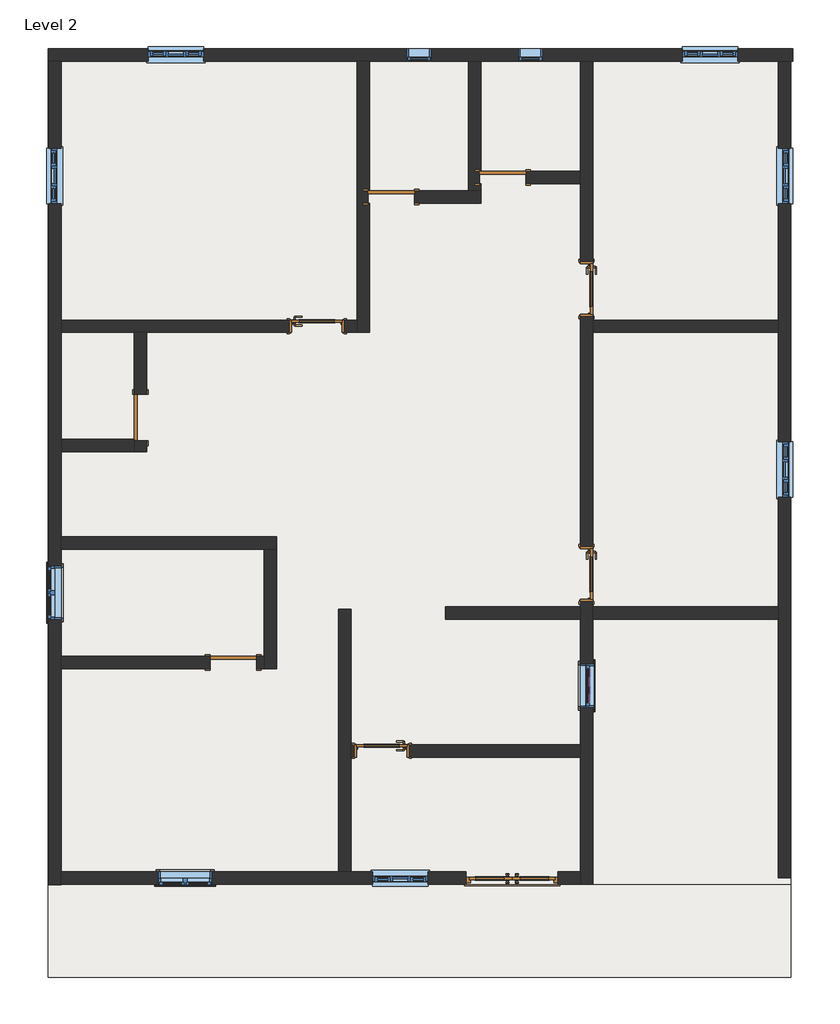
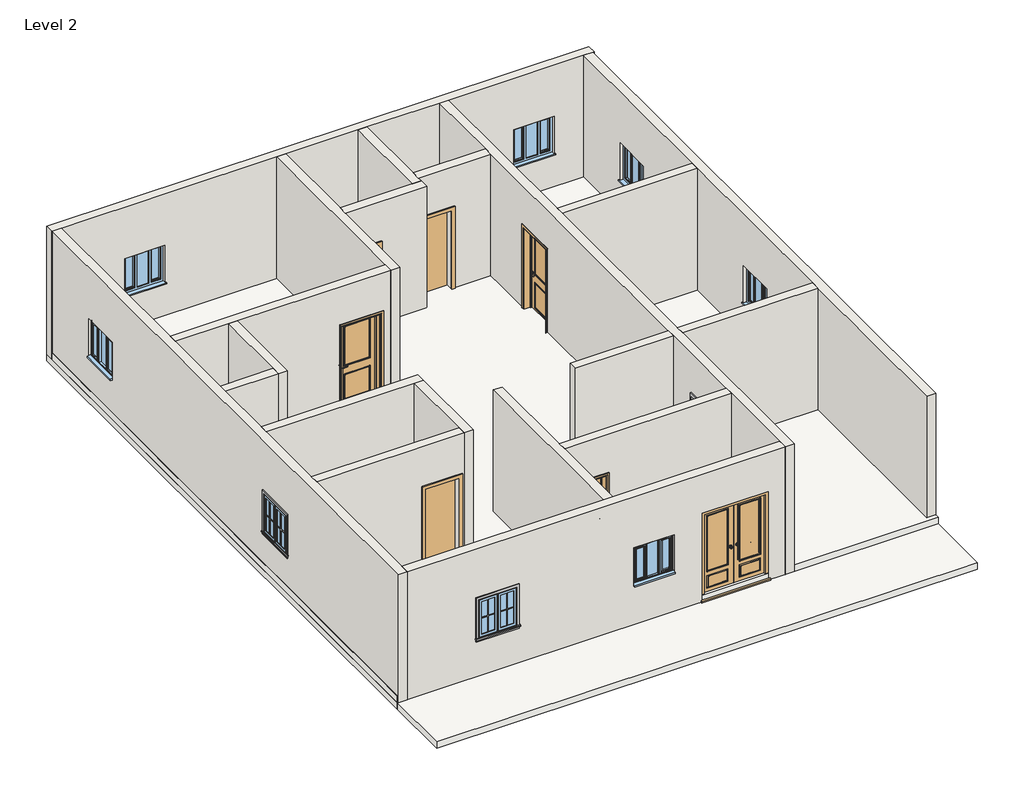
# One storey, incomplete: 19 walls, 12 proxies, 11 windows, 9 doors, 2 slabs, 1 roof.
"""IFC4 building model written with IfcOpenShell, lengths in millimetres."""

from ifc_helpers import new_model, si_unit, frame, origin, place, context, project, spatial, polyline, outline, extrude, faceted_brep, transform, mapped, element, save
from components import muntin_pattern_2x2_muntin_pattern_2x2_b3fe6957, muntin_pattern_2x2_muntin_pattern_2x2_3e0ecaf2, muntin_pattern_2x2_muntin_pattern_2x2_5f474966, trim_window_exterior_flat_with_sill_41619996, trim_window_exterior_flat_with_sill_68241f6a, trim_window_interior_flat_picture_frame_51c85655, trim_window_interior_flat_picture_frame_d3d93820, doors_extdbl_w_glazing_bars_2_1510x2110mm_e5cd3545, doors_extdbl_w_glazing_bars_2_1510x2110mm_b3535315, doors_intsgl_w_transome_910x2110mm_1071bad6, doors_intsgl_w_transome_910x2110mm_0d7ac49b, door_fadea3f2, door_53b1b562, window_085f26e1, window_c29befe5, window_4d695ea9, windows_tpl_plain_910x910mm_84e79c20

model = new_model("IFC4")

# Units and contexts
model_context = context("Model", 3, world=origin())
ifc_project = project(units=[si_unit("LENGTHUNIT", "METRE", prefix="MILLI")], contexts=[model_context])

# Site, building, storey
site = spatial("IfcSite", under=ifc_project)
building = spatial("IfcBuilding", under=site)
storey = spatial("IfcBuildingStorey", under=building, Name="Level 2", Elevation=3048.0)

# Proxies
placement = place(None, origin())
muntin_pattern_2x2_muntin_pattern_2x2_shape = muntin_pattern_2x2_muntin_pattern_2x2_b3fe6957(model_context)
element("IfcBuildingElementProxy", 1, Name="Muntin Pattern_2x2 : Muntin Pattern_2x2", ObjectType="Muntin Pattern_2x2 : Muntin Pattern_2x2", at=placement, inside=storey, context=model_context, shape_type="MappedRepresentation", body=[
    mapped(muntin_pattern_2x2_muntin_pattern_2x2_shape, transform((-4444.3565281, -6259.9254533, 4032.25), x_axis=(-1.0, 0.0, 0.0), y_axis=(0.0, -1.0, 0.0), z_axis=(0.0, 0.0, 1.0))),
])
element("IfcBuildingElementProxy", 2, Name="Muntin Pattern_2x2 : Muntin Pattern_2x2", ObjectType="Muntin Pattern_2x2 : Muntin Pattern_2x2", at=placement, inside=storey, context=model_context, shape_type="MappedRepresentation", body=[
    mapped(muntin_pattern_2x2_muntin_pattern_2x2_shape, transform((-6884.3440281, -1708.5629533, 4032.25), x_axis=(0.0, 1.0, 0.0), y_axis=(-1.0, 0.0, 0.0), z_axis=(0.0, 0.0, 1.0))),
])
muntin_pattern_2x2_muntin_pattern_2x2_2_shape = muntin_pattern_2x2_muntin_pattern_2x2_3e0ecaf2(model_context)
element("IfcBuildingElementProxy", 3, Name="Muntin Pattern_2x2 : Muntin Pattern_2x2", ObjectType="Muntin Pattern_2x2 : Muntin Pattern_2x2", at=placement, inside=storey, context=model_context, shape_type="MappedRepresentation", body=[
    mapped(muntin_pattern_2x2_muntin_pattern_2x2_2_shape, transform((-4872.9815281, -6259.9254533, 4032.25), x_axis=(1.0, 0.0, 0.0), y_axis=(0.0, 1.0, 0.0), z_axis=(0.0, 0.0, 1.0))),
])
element("IfcBuildingElementProxy", 4, Name="Muntin Pattern_2x2 : Muntin Pattern_2x2", ObjectType="Muntin Pattern_2x2 : Muntin Pattern_2x2", at=placement, inside=storey, context=model_context, shape_type="MappedRepresentation", body=[
    mapped(muntin_pattern_2x2_muntin_pattern_2x2_2_shape, transform((-6884.3440281, -1279.9379533, 4032.25), x_axis=(0.0, -1.0, 0.0), y_axis=(1.0, 0.0, 0.0), z_axis=(0.0, 0.0, 1.0))),
])
muntin_pattern_2x2_muntin_pattern_2x2_3_shape = muntin_pattern_2x2_muntin_pattern_2x2_5f474966(model_context)
element("IfcBuildingElementProxy", 5, Name="Muntin Pattern_2x2 : Muntin Pattern_2x2", ObjectType="Muntin Pattern_2x2 : Muntin Pattern_2x2", at=placement, inside=storey, context=model_context, shape_type="MappedRepresentation", body=[
    mapped(muntin_pattern_2x2_muntin_pattern_2x2_3_shape, transform((1989.809459, -3018.2504533, 4568.825), x_axis=(0.0, -1.0, 0.0), y_axis=(1.0, 0.0, 0.0), z_axis=(0.0, 0.0, 1.0))),
])
element("IfcBuildingElementProxy", 6, Name="Muntin Pattern_2x2 : Muntin Pattern_2x2", ObjectType="Muntin Pattern_2x2 : Muntin Pattern_2x2", at=placement, inside=storey, context=model_context, shape_type="MappedRepresentation", body=[
    mapped(muntin_pattern_2x2_muntin_pattern_2x2_3_shape, transform((1945.359459, -3018.2504533, 4038.6), x_axis=(0.0, -1.0, 0.0), y_axis=(1.0, 0.0, 0.0), z_axis=(0.0, 0.0, 1.0))),
])
trim_window_exterior_flat_with_sill_shape = trim_window_exterior_flat_with_sill_41619996(model_context)
element("IfcBuildingElementProxy", 7, Name="Trim-Window-Exterior-Flat : with Sill", ObjectType="Trim-Window-Exterior-Flat : with Sill", at=placement, inside=storey, context=model_context, shape_type="MappedRepresentation", body=[
    mapped(trim_window_exterior_flat_with_sill_shape, transform((-4658.6690281, -6269.4504533, 4876.8), x_axis=(1.0, 0.0, 0.0), y_axis=(0.0, 0.0, 1.0), z_axis=(0.0, -1.0, 0.0))),
])
element("IfcBuildingElementProxy", 8, Name="Trim-Window-Exterior-Flat : with Sill", ObjectType="Trim-Window-Exterior-Flat : with Sill", at=placement, inside=storey, context=model_context, shape_type="MappedRepresentation", body=[
    mapped(trim_window_exterior_flat_with_sill_shape, transform((-6893.8690281, -1494.2504533, 4876.8), x_axis=(0.0, -1.0, 0.0), y_axis=(0.0, 0.0, 1.0), z_axis=(-1.0, 0.0, 0.0))),
])
trim_window_exterior_flat_with_sill_2_shape = trim_window_exterior_flat_with_sill_68241f6a(model_context)
element("IfcBuildingElementProxy", 9, Name="Trim-Window-Exterior-Flat : with Sill", ObjectType="Trim-Window-Exterior-Flat : with Sill", at=placement, inside=storey, context=model_context, shape_type="MappedRepresentation", body=[
    mapped(trim_window_exterior_flat_with_sill_2_shape, transform((2024.734459, -3018.2504533, 5130.8), x_axis=(0.0, 1.0, 0.0), y_axis=(0.0, 0.0, 1.0), z_axis=(1.0, 0.0, 0.0))),
])
trim_window_interior_flat_picture_frame_shape = trim_window_interior_flat_picture_frame_51c85655(model_context)
element("IfcBuildingElementProxy", 10, Name="Trim-Window-Interior-Flat : Picture Frame", ObjectType="Trim-Window-Interior-Flat : Picture Frame", at=placement, inside=storey, context=model_context, shape_type="MappedRepresentation", body=[
    mapped(trim_window_interior_flat_picture_frame_shape, transform((-4658.6690281, -6066.2504533, 4876.8), x_axis=(-1.0, 0.0, 0.0), y_axis=(0.0, 0.0, 1.0), z_axis=(0.0, 1.0, 0.0))),
])
element("IfcBuildingElementProxy", 11, Name="Trim-Window-Interior-Flat : Picture Frame", ObjectType="Trim-Window-Interior-Flat : Picture Frame", at=placement, inside=storey, context=model_context, shape_type="MappedRepresentation", body=[
    mapped(trim_window_interior_flat_picture_frame_shape, transform((-6690.6690281, -1494.2504533, 4876.8), x_axis=(0.0, 1.0, 0.0), y_axis=(0.0, 0.0, 1.0), z_axis=(1.0, 0.0, 0.0))),
])
trim_window_interior_flat_picture_frame_2_shape = trim_window_interior_flat_picture_frame_d3d93820(model_context)
element("IfcBuildingElementProxy", 12, Name="Trim-Window-Interior-Flat : Picture Frame", ObjectType="Trim-Window-Interior-Flat : Picture Frame", at=placement, inside=storey, context=model_context, shape_type="MappedRepresentation", body=[
    mapped(trim_window_interior_flat_picture_frame_2_shape, transform((1821.534459, -3018.2504533, 5130.8), x_axis=(0.0, -1.0, 0.0), y_axis=(0.0, 0.0, 1.0), z_axis=(-1.0, 0.0, 0.0))),
])

# Doors
doors_extdbl_w_glazing_bars_2_1510x2110mm_shape = doors_extdbl_w_glazing_bars_2_1510x2110mm_e5cd3545(model_context)
doors_extdbl_w_glazing_bars_2_1510x2110mm_2_shape = doors_extdbl_w_glazing_bars_2_1510x2110mm_b3535315(model_context)
element("IfcDoor", 13, ObjectType="Doors_ExtDbl_w-Glazing_Bars_2 : 1510x2110mm", at=placement, inside=storey, context=model_context, shape_type="MappedRepresentation", body=[
    mapped(doors_extdbl_w_glazing_bars_2_1510x2110mm_shape, transform((703.934459, -6167.8504533, 3048.0), x_axis=(-1.0, 0.0, 0.0), y_axis=(0.0, -1.0, 0.0), z_axis=(0.0, 0.0, 1.0))),
    mapped(doors_extdbl_w_glazing_bars_2_1510x2110mm_2_shape, transform((703.934459, -6167.8504533, 3048.0), x_axis=(-1.0, 0.0, 0.0), y_axis=(0.0, -1.0, 0.0), z_axis=(0.0, 0.0, 1.0))),
])
doors_intsgl_w_transome_910x2110mm_shape = doors_intsgl_w_transome_910x2110mm_1071bad6(model_context)
element("IfcDoor", 14, ObjectType="Doors_IntSgl_w-Transome : 910x2110mm", at=placement, inside=storey, context=model_context, shape_type="MappedRepresentation", body=[
    mapped(doors_intsgl_w_transome_910x2110mm_shape, transform((-1432.8690281, -4085.0504533, 3048.0), x_axis=(-1.0, 0.0, 0.0), y_axis=(0.0, -1.0, 0.0), z_axis=(0.0, 0.0, 1.0))),
])
doors_intsgl_w_transome_910x2110mm_2_shape = doors_intsgl_w_transome_910x2110mm_0d7ac49b(model_context)
element("IfcDoor", 15, ObjectType="Doors_IntSgl_w-Transome : 910x2110mm", at=placement, inside=storey, context=model_context, shape_type="MappedRepresentation", body=[
    mapped(doors_intsgl_w_transome_910x2110mm_2_shape, transform((-2499.6690281, 2874.5495467, 3048.0), x_axis=(1.0, 0.0, 0.0), y_axis=(0.0, 1.0, 0.0), z_axis=(0.0, 0.0, 1.0))),
])
element("IfcDoor", 16, ObjectType="Doors_IntSgl_w-Transome : 910x2110mm", at=placement, inside=storey, context=model_context, shape_type="MappedRepresentation", body=[
    mapped(doors_intsgl_w_transome_910x2110mm_2_shape, transform((1923.134459, 3484.1495467, 3048.0), x_axis=(0.0, -1.0, 0.0), y_axis=(1.0, 0.0, 0.0), z_axis=(0.0, 0.0, 1.0))),
])
element("IfcDoor", 17, ObjectType="Doors_IntSgl_w-Transome : 910x2110mm", at=placement, inside=storey, context=model_context, shape_type="MappedRepresentation", body=[
    mapped(doors_intsgl_w_transome_910x2110mm_2_shape, transform((1923.134459, -1189.4504533, 3048.0), x_axis=(0.0, -1.0, 0.0), y_axis=(1.0, 0.0, 0.0), z_axis=(0.0, 0.0, 1.0))),
])
door_shape = door_fadea3f2(model_context)
element("IfcDoor", 18, ObjectType="Single-Flush : 30\" x 80\"", at=placement, inside=storey, context=model_context, shape_type="MappedRepresentation", body=[
    mapped(door_shape, transform((-3871.2690281, -2637.2504533, 3048.0), x_axis=(1.0, 0.0, 0.0), y_axis=(0.0, 1.0, 0.0), z_axis=(0.0, 0.0, 1.0))),
])
door_2_shape = door_53b1b562(model_context)
element("IfcDoor", 19, ObjectType="Single-Flush : 30\" x 80\"", at=placement, inside=storey, context=model_context, shape_type="MappedRepresentation", body=[
    mapped(door_2_shape, transform((-5395.2690281, 1375.9495467, 3048.0), x_axis=(0.0, -1.0, 0.0), y_axis=(1.0, 0.0, 0.0), z_axis=(0.0, 0.0, 1.0))),
])
element("IfcDoor", 20, ObjectType="Single-Flush : 30\" x 80\"", at=placement, inside=storey, context=model_context, shape_type="MappedRepresentation", body=[
    mapped(door_2_shape, transform((-1280.4690281, 4995.4495467, 3048.0), x_axis=(-1.0, 0.0, 0.0), y_axis=(0.0, -1.0, 0.0), z_axis=(0.0, 0.0, 1.0))),
])
element("IfcDoor", 21, ObjectType="Single-Flush : 30\" x 80\"", at=placement, inside=storey, context=model_context, shape_type="MappedRepresentation", body=[
    mapped(door_2_shape, transform((548.3309719, 5312.9495467, 3048.0), x_axis=(-1.0, 0.0, 0.0), y_axis=(0.0, -1.0, 0.0), z_axis=(0.0, 0.0, 1.0))),
])

# Roof
element("IfcRoof", 22, ObjectType="Generic - 12\"", at=placement, inside=storey, context=model_context, shape_type="SweptSolid", body=[
    extrude(outline(polyline([(-6906.5690281, 7421.1495467), (5272.7309719, 7421.1495467), (5272.7309719, -6269.4504533), (-6906.5690281, -6269.4504533), (-6906.5690281, 7421.1495467)])), frame((0.0, 0.0, 3048.0), z_axis=(0.0, 0.0, 1.0), x_axis=(1.0, 0.0, 0.0)), (0.0, 0.0, 1.0), 152.4),
])

# Slabs
element("IfcSlab", 23, ObjectType="Generic - 12\"", at=placement, inside=storey, context=model_context, shape_type="SweptSolid", body=[
    extrude(outline(polyline([(5272.7309719, 7421.1495467), (5272.7309719, -6269.4504533), (-6906.5690281, -6269.4504533), (-6906.5690281, 7421.1495467), (5272.7309719, 7421.1495467)])), frame((0.0, 0.0, 2895.6), z_axis=(0.0, 0.0, 1.0), x_axis=(1.0, 0.0, 0.0)), (0.0, 0.0, 1.0), 152.4),
])
element("IfcSlab", 24, ObjectType="Generic - 12\"", at=placement, inside=storey, context=model_context, shape_type="SweptSolid", body=[
    extrude(outline(polyline([(5272.7309719, -6269.4504533), (5272.7309719, -7799.0240652), (-6906.5690281, -7799.0240652), (-6906.5690281, -6269.4504533), (5272.7309719, -6269.4504533)])), frame((0.0, 0.0, 2895.6), z_axis=(0.0, 0.0, 1.0), x_axis=(1.0, 0.0, 0.0)), (0.0, 0.0, 1.0), 152.4),
])

# Walls
element("IfcWall", 25, ObjectType="4.5\" p", at=placement, inside=storey, context=model_context, shape_type="Brep", body=[
    faceted_brep([(-1839.2690281, 7217.9495467, 3048.0), (-1839.2690281, 2976.1495467, 3048.0), (-1839.2690281, 2772.9495467, 3048.0), (-1839.2690281, 2772.9495467, 6096.0), (-1839.2690281, 2976.1495467, 6096.0), (-1839.2690281, 7217.9495467, 6096.0), (-1636.0690281, 7217.9495467, 6096.0), (-1636.0690281, 5097.0495467, 6096.0), (-1636.0690281, 4893.8495467, 6096.0), (-1636.0690281, 2772.9495467, 6096.0), (-1636.0690281, 2772.9495467, 3048.0), (-1636.0690281, 4893.8495467, 3048.0), (-1636.0690281, 4893.8495467, 5080.0), (-1636.0690281, 5097.0495467, 5080.0), (-1636.0690281, 5097.0495467, 3048.0), (-1636.0690281, 7217.9495467, 3048.0), (-1661.4690281, 5097.0495467, 3048.0), (-1661.4690281, 4893.8495467, 3048.0), (-1661.4690281, 5097.0495467, 5080.0), (-1661.4690281, 4893.8495467, 5080.0)], [[[0, 1, 2, 3, 4, 5]], [[6, 7, 8, 9, 10, 11, 12, 13, 14, 15]], [[2, 1, 0, 15, 14, 16, 17, 11, 10]], [[5, 4, 3, 9, 8, 7, 6]], [[0, 5, 6, 15]], [[3, 2, 10, 9]], [[18, 16, 14, 13]], [[17, 19, 12, 11]], [[19, 18, 13, 12]], [[16, 18, 19, 17]]]),
])
element("IfcWall", 26, ObjectType="4.5\" p", at=placement, inside=storey, context=model_context, shape_type="Brep", body=[
    faceted_brep([(-1839.2690281, 2772.9495467, 6096.0), (-5293.6690281, 2772.9495467, 6096.0), (-5496.8690281, 2772.9495467, 6096.0), (-6690.6690281, 2772.9495467, 6096.0), (-6690.6690281, 2772.9495467, 3048.0), (-5496.8690281, 2772.9495467, 3048.0), (-5293.6690281, 2772.9495467, 3048.0), (-2954.6690281, 2772.9495467, 3048.0), (-2954.6690281, 2772.9495467, 5158.0), (-2044.6690281, 2772.9495467, 5158.0), (-2044.6690281, 2772.9495467, 3048.0), (-1839.2690281, 2772.9495467, 3048.0), (-6690.6690281, 2976.1495467, 6096.0), (-1839.2690281, 2976.1495467, 6096.0), (-1839.2690281, 2976.1495467, 3048.0), (-2044.6690281, 2976.1495467, 3048.0), (-2044.6690281, 2976.1495467, 5158.0), (-2954.6690281, 2976.1495467, 5158.0), (-2954.6690281, 2976.1495467, 3048.0), (-6690.6690281, 2976.1495467, 3048.0)], [[[0, 1, 2, 3, 4, 5, 6, 7, 8, 9, 10, 11]], [[12, 13, 14, 15, 16, 17, 18, 19]], [[4, 19, 18, 7, 6, 5]], [[14, 11, 10, 15]], [[3, 2, 1, 0, 13, 12]], [[0, 11, 14, 13]], [[4, 3, 12, 19]], [[9, 16, 15, 10]], [[16, 9, 8, 17]], [[17, 8, 7, 18]]]),
])
element("IfcWall", 27, ObjectType="4.5\" p", at=placement, inside=storey, context=model_context, shape_type="Brep", body=[
    faceted_brep([(-5496.8690281, 994.9495467, 5080.0), (-5496.8690281, 994.9495467, 3048.0), (-5496.8690281, 817.1495467, 3048.0), (-5496.8690281, 817.1495467, 6096.0), (-5496.8690281, 1020.3495467, 6096.0), (-5496.8690281, 2772.9495467, 6096.0), (-5496.8690281, 2772.9495467, 3048.0), (-5496.8690281, 1756.9495467, 3048.0), (-5496.8690281, 1756.9495467, 5080.0), (-5293.6690281, 817.1495467, 3048.0), (-5293.6690281, 994.9495467, 3048.0), (-5293.6690281, 994.9495467, 5080.0), (-5293.6690281, 1756.9495467, 5080.0), (-5293.6690281, 1756.9495467, 3048.0), (-5293.6690281, 2772.9495467, 3048.0), (-5293.6690281, 2772.9495467, 6096.0), (-5293.6690281, 817.1495467, 6096.0)], [[[0, 1, 2, 3, 4, 5, 6, 7, 8]], [[9, 10, 11, 12, 13, 14, 15, 16]], [[7, 6, 14, 13]], [[2, 1, 10, 9]], [[5, 4, 3, 16, 15]], [[6, 5, 15, 14]], [[3, 2, 9, 16]], [[11, 10, 1, 0]], [[12, 11, 0, 8]], [[13, 12, 8, 7]]]),
])
element("IfcWall", 28, ObjectType="4.5\" p", at=placement, inside=storey, context=model_context, shape_type="SweptSolid", body=[
    extrude(outline(polyline([(-5496.8690281, 817.1495467), (-6690.6690281, 817.1495467), (-6690.6690281, 1020.3495467), (-5496.8690281, 1020.3495467), (-5496.8690281, 817.1495467)])), frame((0.0, 0.0, 3048.0), z_axis=(0.0, 0.0, 1.0), x_axis=(1.0, 0.0, 0.0)), (0.0, 0.0, 1.0), 3048.0),
])
element("IfcWall", 29, ObjectType="4.5\" p", at=placement, inside=storey, context=model_context, shape_type="Brep", body=[
    faceted_brep([(-6690.6690281, -783.0504533, 3048.0), (-3363.2690281, -783.0504533, 3048.0), (-3160.0690281, -783.0504533, 3048.0), (-3160.0690281, -783.0504533, 6096.0), (-3363.2690281, -783.0504533, 6096.0), (-6690.6690281, -783.0504533, 6096.0), (-6690.6690281, -579.8504533, 3048.0), (-6690.6690281, -579.8504533, 6096.0), (-3160.0690281, -579.8504533, 6096.0), (-3160.0690281, -579.8504533, 3048.0)], [[[0, 1, 2, 3, 4, 5]], [[6, 7, 8, 9]], [[2, 1, 0, 6, 9]], [[5, 4, 3, 8, 7]], [[0, 5, 7, 6]], [[3, 2, 9, 8]]]),
])
element("IfcWall", 30, ObjectType="4.5\" p", at=placement, inside=storey, context=model_context, shape_type="Brep", body=[
    faceted_brep([(-3363.2690281, -783.0504533, 3048.0), (-3363.2690281, -2535.6504533, 3048.0), (-3363.2690281, -2738.8504533, 3048.0), (-3363.2690281, -2738.8504533, 6096.0), (-3363.2690281, -2535.6504533, 6096.0), (-3363.2690281, -783.0504533, 6096.0), (-3160.0690281, -783.0504533, 3048.0), (-3160.0690281, -783.0504533, 6096.0), (-3160.0690281, -2738.8504533, 6096.0), (-3160.0690281, -2738.8504533, 3048.0)], [[[0, 1, 2, 3, 4, 5]], [[6, 7, 8, 9]], [[2, 1, 0, 6, 9]], [[5, 4, 3, 8, 7]], [[0, 5, 7, 6]], [[3, 2, 9, 8]]]),
])
element("IfcWall", 31, ObjectType="4.5\" p", at=placement, inside=storey, context=model_context, shape_type="SweptSolid", body=[
    extrude(outline(polyline([(5080.0, -3490.2690281), (3048.0, -3490.2690281), (3048.0, -3363.2690281), (6096.0, -3363.2690281), (6096.0, -6690.6690281), (3048.0, -6690.6690281), (3048.0, -4252.2690281), (5080.0, -4252.2690281), (5080.0, -3490.2690281)])), frame((0.0, -2738.8504533, 0.0), z_axis=(0.0, 1.0, 0.0), x_axis=(0.0, 0.0, 1.0)), (0.0, 0.0, 1.0), 203.2),
])
element("IfcWall", 32, ObjectType="4.5\" p", at=placement, inside=storey, context=model_context, shape_type="Brep", body=[
    faceted_brep([(192.7309719, 4893.8495467, 6096.0), (-1636.0690281, 4893.8495467, 6096.0), (-1636.0690281, 4893.8495467, 5080.0), (-899.4690281, 4893.8495467, 5080.0), (-899.4690281, 4893.8495467, 3048.0), (192.7309719, 4893.8495467, 3048.0), (-1636.0690281, 5097.0495467, 6096.0), (-10.4690281, 5097.0495467, 6096.0), (192.7309719, 5097.0495467, 6096.0), (192.7309719, 5097.0495467, 3048.0), (-10.4690281, 5097.0495467, 3048.0), (-899.4690281, 5097.0495467, 3048.0), (-899.4690281, 5097.0495467, 5080.0), (-1636.0690281, 5097.0495467, 5080.0)], [[[0, 1, 2, 3, 4, 5]], [[6, 7, 8, 9, 10, 11, 12, 13]], [[9, 5, 4, 11, 10]], [[1, 0, 8, 7, 6]], [[1, 6, 13, 2]], [[0, 5, 9, 8]], [[12, 3, 2, 13]], [[3, 12, 11, 4]]]),
])
element("IfcWall", 33, ObjectType="4.5\" p", at=placement, inside=storey, context=model_context, shape_type="Brep", body=[
    faceted_brep([(-10.4690281, 7217.9495467, 3048.0), (-10.4690281, 5097.0495467, 3048.0), (-10.4690281, 5097.0495467, 6096.0), (-10.4690281, 7217.9495467, 6096.0), (192.7309719, 7217.9495467, 6096.0), (192.7309719, 5414.5495467, 6096.0), (192.7309719, 5211.3495467, 6096.0), (192.7309719, 5097.0495467, 6096.0), (192.7309719, 5097.0495467, 3048.0), (192.7309719, 5211.3495467, 3048.0), (192.7309719, 5211.3495467, 5080.0), (192.7309719, 5414.5495467, 5080.0), (192.7309719, 5414.5495467, 3048.0), (192.7309719, 7217.9495467, 3048.0), (167.3309719, 5414.5495467, 3048.0), (167.3309719, 5211.3495467, 3048.0), (167.3309719, 5414.5495467, 5080.0), (167.3309719, 5211.3495467, 5080.0)], [[[0, 1, 2, 3]], [[4, 5, 6, 7, 8, 9, 10, 11, 12, 13]], [[1, 0, 13, 12, 14, 15, 9, 8]], [[3, 2, 7, 6, 5, 4]], [[2, 1, 8, 7]], [[0, 3, 4, 13]], [[16, 14, 12, 11]], [[15, 17, 10, 9]], [[17, 16, 11, 10]], [[14, 16, 17, 15]]]),
])
element("IfcWall", 34, ObjectType="4.5\" p", at=placement, inside=storey, context=model_context, shape_type="Brep", body=[
    faceted_brep([(1821.534459, -6269.4504533, 6096.0), (1821.534459, -6066.2504533, 6096.0), (1821.534459, -4186.6504533, 6096.0), (1821.534459, -3983.4504533, 6096.0), (1821.534459, -1926.0504533, 6096.0), (1821.534459, -1722.8504533, 6096.0), (1821.534459, 5211.3495467, 6096.0), (1821.534459, 5414.5495467, 6096.0), (1821.534459, 7217.9495467, 6096.0), (1821.534459, 7217.9495467, 3048.0), (1821.534459, 5414.5495467, 3048.0), (1821.534459, 5211.3495467, 3048.0), (1821.534459, 3939.1495467, 3048.0), (1821.534459, 3939.1495467, 5158.0), (1821.534459, 3029.1495467, 5158.0), (1821.534459, 3029.1495467, 3048.0), (1821.534459, -734.4504533, 3048.0), (1821.534459, -734.4504533, 5158.0), (1821.534459, -1644.4504533, 5158.0), (1821.534459, -1644.4504533, 3048.0), (1821.534459, -1722.8504533, 3048.0), (1821.534459, -1926.0504533, 3048.0), (1821.534459, -3983.4504533, 3048.0), (1821.534459, -4186.6504533, 3048.0), (1821.534459, -6066.2504533, 3048.0), (1821.534459, -6269.4504533, 3048.0), (1821.534459, -2662.6504533, 5130.8), (1821.534459, -3373.8504533, 5130.8), (1821.534459, -3373.8504533, 3962.4), (1821.534459, -2662.6504533, 3962.4), (2024.734459, 7217.9495467, 6096.0), (2024.734459, 2976.1495467, 6096.0), (2024.734459, 2772.9495467, 6096.0), (2024.734459, -1722.8504533, 6096.0), (2024.734459, -1926.0504533, 6096.0), (2024.734459, -6269.4504533, 6096.0), (2024.734459, -6269.4504533, 3048.0), (2024.734459, -1926.0504533, 3048.0), (2024.734459, -1722.8504533, 3048.0), (2024.734459, -1644.4504533, 3048.0), (2024.734459, -1644.4504533, 5158.0), (2024.734459, -734.4504533, 5158.0), (2024.734459, -734.4504533, 3048.0), (2024.734459, 2772.9495467, 3048.0), (2024.734459, 2976.1495467, 3048.0), (2024.734459, 3029.1495467, 3048.0), (2024.734459, 3029.1495467, 5158.0), (2024.734459, 3939.1495467, 5158.0), (2024.734459, 3939.1495467, 3048.0), (2024.734459, 7217.9495467, 3048.0), (2024.734459, -2662.6504533, 5130.8), (2024.734459, -2662.6504533, 3962.4), (2024.734459, -3373.8504533, 3962.4), (2024.734459, -3373.8504533, 5130.8)], [[[0, 1, 2, 3, 4, 5, 6, 7, 8, 9, 10, 11, 12, 13, 14, 15, 16, 17, 18, 19, 20, 21, 22, 23, 24, 25], [26, 27, 28, 29]], [[30, 31, 32, 33, 34, 35, 36, 37, 38, 39, 40, 41, 42, 43, 44, 45, 46, 47, 48, 49], [50, 51, 52, 53]], [[9, 49, 48, 12, 11, 10]], [[15, 45, 44, 43, 42, 16]], [[36, 25, 24, 23, 22, 21, 20, 19, 39, 38, 37]], [[8, 7, 6, 5, 4, 3, 2, 1, 0, 35, 34, 33, 32, 31, 30]], [[9, 8, 30, 49]], [[14, 46, 45, 15]], [[46, 14, 13, 47]], [[47, 13, 12, 48]], [[18, 40, 39, 19]], [[40, 18, 17, 41]], [[41, 17, 16, 42]], [[0, 25, 36, 35]], [[51, 50, 26, 29]], [[52, 51, 29, 28]], [[53, 52, 28, 27]], [[50, 53, 27, 26]]]),
])
element("IfcWall", 35, ObjectType="4.5\" p", at=placement, inside=storey, context=model_context, shape_type="SweptSolid", body=[
    extrude(outline(polyline([(-391.4690281, -1926.0504533), (-391.4690281, -1722.8504533), (1821.534459, -1722.8504533), (1821.534459, -1926.0504533), (-391.4690281, -1926.0504533)])), frame((0.0, 0.0, 3048.0), z_axis=(0.0, 0.0, 1.0), x_axis=(1.0, 0.0, 0.0)), (0.0, 0.0, 1.0), 3048.0),
    extrude(outline(polyline([(5069.5309719, -1722.8504533), (5069.5309719, -1926.0504533), (2024.734459, -1926.0504533), (2024.734459, -1722.8504533), (5069.5309719, -1722.8504533)])), frame((0.0, 0.0, 3048.0), z_axis=(0.0, 0.0, 1.0), x_axis=(1.0, 0.0, 0.0)), (0.0, 0.0, 1.0), 3048.0),
])
element("IfcWall", 36, ObjectType="4.5\" p", at=placement, inside=storey, context=model_context, shape_type="SweptSolid", body=[
    extrude(outline(polyline([(5069.5309719, 2772.9495467), (2024.734459, 2772.9495467), (2024.734459, 2976.1495467), (5069.5309719, 2976.1495467), (5069.5309719, 2772.9495467)])), frame((0.0, 0.0, 3048.0), z_axis=(0.0, 0.0, 1.0), x_axis=(1.0, 0.0, 0.0)), (0.0, 0.0, 1.0), 3048.0),
])
element("IfcWall", 37, ObjectType="4.5\" p", at=placement, inside=storey, context=model_context, shape_type="SweptSolid", body=[
    extrude(outline(polyline([(6096.0, 1821.534459), (6096.0, 192.7309719), (5080.0, 192.7309719), (5080.0, 929.3309719), (3048.0, 929.3309719), (3048.0, 1821.534459), (6096.0, 1821.534459)])), frame((0.0, 5211.3495467, 0.0), z_axis=(0.0, 1.0, 0.0), x_axis=(0.0, 0.0, 1.0)), (0.0, 0.0, 1.0), 203.2),
])
element("IfcWall", 38, ObjectType="4.5\" p", at=placement, inside=storey, context=model_context, shape_type="Brep", body=[
    faceted_brep([(-1940.8690281, -6066.2504533, 3048.0), (-1940.8690281, -4186.6504533, 3048.0), (-1940.8690281, -3983.4504533, 3048.0), (-1940.8690281, -1760.9504533, 3048.0), (-1940.8690281, -1760.9504533, 6096.0), (-1940.8690281, -3983.4504533, 6096.0), (-1940.8690281, -4186.6504533, 6096.0), (-1940.8690281, -6066.2504533, 6096.0), (-2144.0690281, -6066.2504533, 3048.0), (-2144.0690281, -6066.2504533, 6096.0), (-2144.0690281, -1760.9504533, 6096.0), (-2144.0690281, -1760.9504533, 3048.0)], [[[0, 1, 2, 3, 4, 5, 6, 7]], [[8, 9, 10, 11]], [[3, 2, 1, 0, 8, 11]], [[4, 3, 11, 10]], [[7, 6, 5, 4, 10, 9]], [[0, 7, 9, 8]]]),
])
element("IfcWall", 39, ObjectType="4.5\" p", at=placement, inside=storey, context=model_context, shape_type="SweptSolid", body=[
    extrude(outline(polyline([(6096.0, 1821.534459), (6096.0, -1940.8690281), (3048.0, -1940.8690281), (3048.0, -1887.8690281), (5158.0, -1887.8690281), (5158.0, -977.8690281), (3048.0, -977.8690281), (3048.0, 1821.534459), (6096.0, 1821.534459)])), frame((0.0, -4186.6504533, 0.0), z_axis=(0.0, 1.0, 0.0), x_axis=(0.0, 0.0, 1.0)), (0.0, 0.0, 1.0), 203.2),
])
element("IfcWall", 40, ObjectType="9\"", at=placement, inside=storey, context=model_context, shape_type="Brep", body=[
    faceted_brep([(5069.5309719, 7217.9495467, 3048.0), (5069.5309719, 2976.1495467, 3048.0), (5069.5309719, 2772.9495467, 3048.0), (5069.5309719, -1722.8504533, 3048.0), (5069.5309719, -1926.0504533, 3048.0), (5069.5309719, -6167.8504533, 3048.0), (5069.5309719, -6167.8504533, 6096.0), (5069.5309719, -1926.0504533, 6096.0), (5069.5309719, -1722.8504533, 6096.0), (5069.5309719, 2772.9495467, 6096.0), (5069.5309719, 2976.1495467, 6096.0), (5069.5309719, 7217.9495467, 6096.0), (5069.5309719, 980.0495467, 4872.4), (5069.5309719, 70.0495467, 4872.4), (5069.5309719, 70.0495467, 3962.4), (5069.5309719, 980.0495467, 3962.4), (5069.5309719, 5793.3495467, 4872.4), (5069.5309719, 4883.3495467, 4872.4), (5069.5309719, 4883.3495467, 3962.4), (5069.5309719, 5793.3495467, 3962.4), (5272.7309719, 7217.9495467, 3048.0), (5272.7309719, 7217.9495467, 6096.0), (5272.7309719, -6167.8504533, 6096.0), (5272.7309719, -6167.8504533, 3048.0), (5272.7309719, 980.0495467, 4872.4), (5272.7309719, 980.0495467, 3962.4), (5272.7309719, 70.0495467, 3962.4), (5272.7309719, 70.0495467, 4872.4), (5272.7309719, 5793.3495467, 4872.4), (5272.7309719, 5793.3495467, 3962.4), (5272.7309719, 4883.3495467, 3962.4), (5272.7309719, 4883.3495467, 4872.4)], [[[0, 1, 2, 3, 4, 5, 6, 7, 8, 9, 10, 11], [12, 13, 14, 15], [16, 17, 18, 19]], [[20, 21, 22, 23], [24, 25, 26, 27], [28, 29, 30, 31]], [[5, 4, 3, 2, 1, 0, 20, 23]], [[6, 5, 23, 22]], [[11, 10, 9, 8, 7, 6, 22, 21]], [[0, 11, 21, 20]], [[25, 24, 12, 15]], [[26, 25, 15, 14]], [[27, 26, 14, 13]], [[24, 27, 13, 12]], [[29, 28, 16, 19]], [[30, 29, 19, 18]], [[31, 30, 18, 17]], [[28, 31, 17, 16]]]),
])
element("IfcWall", 41, ObjectType="9\" wall", at=placement, inside=storey, context=model_context, shape_type="Brep", body=[
    faceted_brep([(-6906.5690281, 7217.9495467, 3048.0), (-6893.8690281, 7217.9495467, 3048.0), (-6690.6690281, 7217.9495467, 3048.0), (-1839.2690281, 7217.9495467, 3048.0), (-1636.0690281, 7217.9495467, 3048.0), (-10.4690281, 7217.9495467, 3048.0), (192.7309719, 7217.9495467, 3048.0), (1821.534459, 7217.9495467, 3048.0), (2024.734459, 7217.9495467, 3048.0), (5069.5309719, 7217.9495467, 3048.0), (5272.7309719, 7217.9495467, 3048.0), (5310.8309719, 7217.9495467, 3048.0), (5310.8309719, 7217.9495467, 6096.0), (5272.7309719, 7217.9495467, 6096.0), (5069.5309719, 7217.9495467, 6096.0), (2024.734459, 7217.9495467, 6096.0), (1821.534459, 7217.9495467, 6096.0), (192.7309719, 7217.9495467, 6096.0), (-10.4690281, 7217.9495467, 6096.0), (-1636.0690281, 7217.9495467, 6096.0), (-1839.2690281, 7217.9495467, 6096.0), (-6690.6690281, 7217.9495467, 6096.0), (-6893.8690281, 7217.9495467, 6096.0), (-6906.5690281, 7217.9495467, 6096.0), (-5266.0690281, 7217.9495467, 4872.4), (-4356.0690281, 7217.9495467, 4872.4), (-4356.0690281, 7217.9495467, 3962.4), (-5266.0690281, 7217.9495467, 3962.4), (3496.9309719, 7217.9495467, 4872.4), (4406.9309719, 7217.9495467, 4872.4), (4406.9309719, 7217.9495467, 3962.4), (3496.9309719, 7217.9495467, 3962.4), (-1026.4690281, 7217.9495467, 4572.0), (-620.0690281, 7217.9495467, 4572.0), (-620.0690281, 7217.9495467, 3962.4), (-1026.4690281, 7217.9495467, 3962.4), (803.9327155, 7217.9495467, 4572.0), (1210.3327155, 7217.9495467, 4572.0), (1210.3327155, 7217.9495467, 3962.4), (803.9327155, 7217.9495467, 3962.4), (-6906.5690281, 7421.1495467, 3048.0), (-6906.5690281, 7421.1495467, 6096.0), (5310.8309719, 7421.1495467, 6096.0), (5310.8309719, 7421.1495467, 3048.0), (-5266.0690281, 7421.1495467, 4872.4), (-5266.0690281, 7421.1495467, 3962.4), (-4356.0690281, 7421.1495467, 3962.4), (-4356.0690281, 7421.1495467, 4872.4), (3496.9309719, 7421.1495467, 4872.4), (3496.9309719, 7421.1495467, 3962.4), (4406.9309719, 7421.1495467, 3962.4), (4406.9309719, 7421.1495467, 4872.4), (-1026.4690281, 7421.1495467, 4572.0), (-1026.4690281, 7421.1495467, 3962.4), (-620.0690281, 7421.1495467, 3962.4), (-620.0690281, 7421.1495467, 4572.0), (803.9327155, 7421.1495467, 4572.0), (803.9327155, 7421.1495467, 3962.4), (1210.3327155, 7421.1495467, 3962.4), (1210.3327155, 7421.1495467, 4572.0)], [[[0, 1, 2, 3, 4, 5, 6, 7, 8, 9, 10, 11, 12, 13, 14, 15, 16, 17, 18, 19, 20, 21, 22, 23], [24, 25, 26, 27], [28, 29, 30, 31], [32, 33, 34, 35], [36, 37, 38, 39]], [[40, 41, 42, 43], [44, 45, 46, 47], [48, 49, 50, 51], [52, 53, 54, 55], [56, 57, 58, 59]], [[11, 10, 9, 8, 7, 6, 5, 4, 3, 2, 1, 0, 40, 43]], [[12, 11, 43, 42]], [[23, 22, 21, 20, 19, 18, 17, 16, 15, 14, 13, 12, 42, 41]], [[0, 23, 41, 40]], [[45, 44, 24, 27]], [[46, 45, 27, 26]], [[47, 46, 26, 25]], [[44, 47, 25, 24]], [[49, 48, 28, 31]], [[50, 49, 31, 30]], [[51, 50, 30, 29]], [[48, 51, 29, 28]], [[53, 52, 32, 35]], [[54, 53, 35, 34]], [[55, 54, 34, 33]], [[52, 55, 33, 32]], [[57, 56, 36, 39]], [[58, 57, 39, 38]], [[59, 58, 38, 37]], [[56, 59, 37, 36]]]),
])
element("IfcWall", 42, ObjectType="9\" wall", at=placement, inside=storey, context=model_context, shape_type="Brep", body=[
    faceted_brep([(-6893.8690281, 7217.9495467, 3048.0), (-6893.8690281, -6282.1504533, 3048.0), (-6893.8690281, -6282.1504533, 6096.0), (-6893.8690281, 7217.9495467, 6096.0), (-6893.8690281, -1062.4504533, 4876.8), (-6893.8690281, -1926.0504533, 4876.8), (-6893.8690281, -1926.0504533, 3962.4), (-6893.8690281, -1062.4504533, 3962.4), (-6893.8690281, 4883.3495467, 4872.4), (-6893.8690281, 4883.3495467, 3962.4), (-6893.8690281, 5793.3495467, 3962.4), (-6893.8690281, 5793.3495467, 4872.4), (-6690.6690281, 7217.9495467, 3048.0), (-6690.6690281, 7217.9495467, 6096.0), (-6690.6690281, 2976.1495467, 6096.0), (-6690.6690281, 2772.9495467, 6096.0), (-6690.6690281, 1020.3495467, 6096.0), (-6690.6690281, 817.1495467, 6096.0), (-6690.6690281, -579.8504533, 6096.0), (-6690.6690281, -783.0504533, 6096.0), (-6690.6690281, -2535.6504533, 6096.0), (-6690.6690281, -2738.8504533, 6096.0), (-6690.6690281, -6066.2504533, 6096.0), (-6690.6690281, -6269.4504533, 6096.0), (-6690.6690281, -6282.1504533, 6096.0), (-6690.6690281, -6282.1504533, 3048.0), (-6690.6690281, -6269.4504533, 3048.0), (-6690.6690281, -6066.2504533, 3048.0), (-6690.6690281, -2738.8504533, 3048.0), (-6690.6690281, -2535.6504533, 3048.0), (-6690.6690281, -783.0504533, 3048.0), (-6690.6690281, -579.8504533, 3048.0), (-6690.6690281, 817.1495467, 3048.0), (-6690.6690281, 1020.3495467, 3048.0), (-6690.6690281, 2772.9495467, 3048.0), (-6690.6690281, 2976.1495467, 3048.0), (-6690.6690281, -1062.4504533, 4876.8), (-6690.6690281, -1062.4504533, 3962.4), (-6690.6690281, -1926.0504533, 3962.4), (-6690.6690281, -1926.0504533, 4876.8), (-6690.6690281, 4883.3495467, 4872.4), (-6690.6690281, 5793.3495467, 4872.4), (-6690.6690281, 5793.3495467, 3962.4), (-6690.6690281, 4883.3495467, 3962.4)], [[[0, 1, 2, 3], [4, 5, 6, 7], [8, 9, 10, 11]], [[12, 13, 14, 15, 16, 17, 18, 19, 20, 21, 22, 23, 24, 25, 26, 27, 28, 29, 30, 31, 32, 33, 34, 35], [36, 37, 38, 39], [40, 41, 42, 43]], [[1, 0, 12, 35, 34, 33, 32, 31, 30, 29, 28, 27, 26, 25]], [[2, 1, 25, 24]], [[3, 2, 24, 23, 22, 21, 20, 19, 18, 17, 16, 15, 14, 13]], [[0, 3, 13, 12]], [[37, 36, 4, 7]], [[38, 37, 7, 6]], [[39, 38, 6, 5]], [[36, 39, 5, 4]], [[9, 8, 40, 43]], [[10, 9, 43, 42]], [[11, 10, 42, 41]], [[8, 11, 41, 40]]]),
])
element("IfcWall", 43, ObjectType="9\" wall", at=placement, inside=storey, context=model_context, shape_type="Brep", body=[
    faceted_brep([(1821.534459, -6269.4504533, 6096.0), (-6690.6690281, -6269.4504533, 6096.0), (-6690.6690281, -6269.4504533, 3048.0), (-51.065541, -6269.4504533, 3048.0), (-51.065541, -6269.4504533, 5158.0), (1458.934459, -6269.4504533, 5158.0), (1458.934459, -6269.4504533, 3048.0), (1821.534459, -6269.4504533, 3048.0), (-5090.4690281, -6269.4504533, 4876.8), (-4226.8690281, -6269.4504533, 4876.8), (-4226.8690281, -6269.4504533, 3962.4), (-5090.4690281, -6269.4504533, 3962.4), (-673.0690281, -6269.4504533, 4872.4), (-673.0690281, -6269.4504533, 3962.4), (-1583.0690281, -6269.4504533, 3962.4), (-1583.0690281, -6269.4504533, 4872.4), (-6690.6690281, -6066.2504533, 6096.0), (-2144.0690281, -6066.2504533, 6096.0), (-1940.8690281, -6066.2504533, 6096.0), (1821.534459, -6066.2504533, 6096.0), (1821.534459, -6066.2504533, 3048.0), (1458.934459, -6066.2504533, 3048.0), (1458.934459, -6066.2504533, 5158.0), (-51.065541, -6066.2504533, 5158.0), (-51.065541, -6066.2504533, 3048.0), (-1940.8690281, -6066.2504533, 3048.0), (-2144.0690281, -6066.2504533, 3048.0), (-6690.6690281, -6066.2504533, 3048.0), (-5090.4690281, -6066.2504533, 4876.8), (-5090.4690281, -6066.2504533, 3962.4), (-4226.8690281, -6066.2504533, 3962.4), (-4226.8690281, -6066.2504533, 4876.8), (-673.0690281, -6066.2504533, 4872.4), (-1583.0690281, -6066.2504533, 4872.4), (-1583.0690281, -6066.2504533, 3962.4), (-673.0690281, -6066.2504533, 3962.4)], [[[0, 1, 2, 3, 4, 5, 6, 7], [8, 9, 10, 11], [12, 13, 14, 15]], [[16, 17, 18, 19, 20, 21, 22, 23, 24, 25, 26, 27], [28, 29, 30, 31], [32, 33, 34, 35]], [[20, 7, 6, 21]], [[2, 27, 26, 25, 24, 3]], [[1, 0, 19, 18, 17, 16]], [[0, 7, 20, 19]], [[2, 1, 16, 27]], [[29, 28, 8, 11]], [[30, 29, 11, 10]], [[31, 30, 10, 9]], [[28, 31, 9, 8]], [[5, 22, 21, 6]], [[22, 5, 4, 23]], [[23, 4, 3, 24]], [[13, 12, 32, 35]], [[14, 13, 35, 34]], [[15, 14, 34, 33]], [[12, 15, 33, 32]]]),
])

# Windows
window_shape = window_085f26e1(model_context)
element("IfcWindow", 44, ObjectType="Fixed : 16\" x 24\"", at=placement, inside=storey, context=model_context, shape_type="MappedRepresentation", body=[
    mapped(window_shape, transform((-861.3690281, 7319.5495467, 3048.0), x_axis=(-1.0, 0.0, 0.0), y_axis=(0.0, -1.0, 0.0), z_axis=(0.0, 0.0, 1.0))),
])
element("IfcWindow", 45, ObjectType="Fixed : 16\" x 24\"", at=placement, inside=storey, context=model_context, shape_type="MappedRepresentation", body=[
    mapped(window_shape, transform((969.0327155, 7319.5495467, 3048.0), x_axis=(-1.0, 0.0, 0.0), y_axis=(0.0, -1.0, 0.0), z_axis=(0.0, 0.0, 1.0))),
])
window_2_shape = window_c29befe5(model_context)
element("IfcWindow", 46, ObjectType="Window-Casement-Double : 34\" x 36\"", at=placement, inside=storey, context=model_context, shape_type="MappedRepresentation", body=[
    mapped(window_2_shape, transform((-4658.6690281, -6167.8504533, 3048.0), x_axis=(-1.0, 0.0, 0.0), y_axis=(0.0, -1.0, 0.0), z_axis=(0.0, 0.0, 1.0))),
])
element("IfcWindow", 47, ObjectType="Window-Casement-Double : 34\" x 36\"", at=placement, inside=storey, context=model_context, shape_type="MappedRepresentation", body=[
    mapped(window_2_shape, transform((-6792.2690281, -1494.2504533, 3048.0), x_axis=(0.0, 1.0, 0.0), y_axis=(-1.0, 0.0, 0.0), z_axis=(0.0, 0.0, 1.0))),
])
window_3_shape = window_4d695ea9(model_context)
element("IfcWindow", 48, ObjectType="Window-Double-Hung : 28\" x 46\"", at=placement, inside=storey, context=model_context, shape_type="MappedRepresentation", body=[
    mapped(window_3_shape, transform((1923.134459, -3018.2504533, 3048.0), x_axis=(0.0, -1.0, 0.0), y_axis=(1.0, 0.0, 0.0), z_axis=(0.0, 0.0, 1.0))),
])
windows_tpl_plain_910x910mm_shape = windows_tpl_plain_910x910mm_84e79c20(model_context)
element("IfcWindow", 49, ObjectType="Windows_Tpl_Plain : 910x910mm", at=placement, inside=storey, context=model_context, shape_type="MappedRepresentation", body=[
    mapped(windows_tpl_plain_910x910mm_shape, transform((-1554.7356948, -6159.3938855, 2762.4), x_axis=(-1.0, 0.0, 0.0), y_axis=(0.0, -1.0, 0.0), z_axis=(0.0, 0.0, 1.0))),
])
element("IfcWindow", 50, ObjectType="Windows_Tpl_Plain : 910x910mm", at=placement, inside=storey, context=model_context, shape_type="MappedRepresentation", body=[
    mapped(windows_tpl_plain_910x910mm_shape, transform((-6783.8124603, 5765.0162133, 2762.4), x_axis=(0.0, 1.0, 0.0), y_axis=(-1.0, 0.0, 0.0), z_axis=(0.0, 0.0, 1.0))),
])
element("IfcWindow", 51, ObjectType="Windows_Tpl_Plain : 910x910mm", at=placement, inside=storey, context=model_context, shape_type="MappedRepresentation", body=[
    mapped(windows_tpl_plain_910x910mm_shape, transform((-4384.4023614, 7311.0929788, 2762.4), x_axis=(1.0, 0.0, 0.0), y_axis=(0.0, 1.0, 0.0), z_axis=(0.0, 0.0, 1.0))),
])
element("IfcWindow", 52, ObjectType="Windows_Tpl_Plain : 910x910mm", at=placement, inside=storey, context=model_context, shape_type="MappedRepresentation", body=[
    mapped(windows_tpl_plain_910x910mm_shape, transform((4378.5976386, 7311.0929788, 2762.4), x_axis=(1.0, 0.0, 0.0), y_axis=(0.0, 1.0, 0.0), z_axis=(0.0, 0.0, 1.0))),
])
element("IfcWindow", 53, ObjectType="Windows_Tpl_Plain : 910x910mm", at=placement, inside=storey, context=model_context, shape_type="MappedRepresentation", body=[
    mapped(windows_tpl_plain_910x910mm_shape, transform((5162.6744041, 98.38288, 2762.4), x_axis=(0.0, -1.0, 0.0), y_axis=(1.0, 0.0, 0.0), z_axis=(0.0, 0.0, 1.0))),
])
element("IfcWindow", 54, ObjectType="Windows_Tpl_Plain : 910x910mm", at=placement, inside=storey, context=model_context, shape_type="MappedRepresentation", body=[
    mapped(windows_tpl_plain_910x910mm_shape, transform((5162.6744041, 4911.68288, 2762.4), x_axis=(0.0, -1.0, 0.0), y_axis=(1.0, 0.0, 0.0), z_axis=(0.0, 0.0, 1.0))),
])

save(model, "model.ifc")

# Revit data of these elements
# Type "Muntin Pattern_2x2 : Muntin Pattern_2x2"
#   Width [instance default] = 4' - 0"
#   Thickness = 0' - 0 1/2"
#   Height [instance default] = 4' - 0"
#   Distance = 0' - 0 3/4"
#   Interior Material [instance default] = none
#   Exterior Material [instance default] = none
#   Default Elevation = 0
# Type "Trim-Window-Exterior-Flat : with Sill"
#   Trim Width = 0' - 2 1/4"
#   Trim Thickness_Picture Frame = 0' - 1 1/4"
#   Trim Thickness_with Sill = 0' - 0 3/4"
#   Sill Thickness = 0' - 1 1/4"
#   Opening Width [instance default] = 2' - 0"
#   Opening Height [instance default] = 3' - 0"
#   Default Elevation = 4' - 0"
#   Sill = yes
#   Picture Frame = no
#   Trim Material [instance default] = none
# Type "Trim-Window-Interior-Flat : Picture Frame"
#   Trim Thickness_Picture Frame = 0' - 1 1/4"
#   Trim Width = 0' - 2 1/4"
#   Trim Thickness_with Sill = 0' - 0 3/4"
#   Sill Thickness = 0' - 1 1/4"
#   Opening Width [instance default] = 2' - 0"
#   Opening Height [instance default] = 3' - 0"
#   Default Elevation = 4' - 0"
#   Sill = no
#   Picture Frame = yes
#   Trim Material [instance default] = none
# Type "Doors_ExtDbl_w-Glazing_Bars_2 : 1510x2110mm"
#   Type Mark = "15"
#   Type Comments = "External Double"
#   Operation = "DoubleDoorSingleSwing"
#   Construction Type Id = "GSP4R"
#   Keynote = "L20"
#   Analytic Construction = "1/8 in Pilkington single glazing"
#   Wrap Layers (Int) from Ext = 0' - 6.98819"
#   Wrap Layers (Ext) from Ext = 0' - 4.03543"
#   Visual Light Transmittance = 0.9
#   Top of Intermediate Rail = 1' - 10.6378"
#   Thickness = 0' - 1.73228"
#   Stile Shutting = 0' - 4.92126"
#   Stile - Top Rail = 0' - 3.93701"
#   Stile - Lock Rail = 0' - 3.93701"
#   Stile - Hanging = 0' - 3.93701"
#   Stile - Bottom Rail = 0' - 6.88976"
#   Solar Heat Gain Coefficient = 0.78
#   Rough Width = 4' - 11.44882"
#   Rough Height = 6' - 11.07087"
#   O/A Frame Width = 0' - 2.51969"
#   Heat Transfer Coefficient (U) = 0.6496 BTU/(h·ft²·°F)
#   Handle Z Distance = 3' - 5.33858"
#   Glazing Thickness = 0' - 0.94488"
#   Glazing Bar Thickness = 0' - 0.7874"
#   FrameWidth = 0' - 1.65354"
#   FrameOffset - External = 0' - 0.98425"
#   FrameDepth = 0' - 3.50394"
#   Door Panel Width = 2' - 3.6378"
#   Door Panel Thickness = 0' - 1.73228"
#   Door Panel Height = 6' - 6.74016"
#   Cill Thickness = 0' - 2.14567"
#   Cill Projection = 0' - 1.1811"
#   Handle X Distance = 0' - 2.95276"
#   Height = 6' - 11.07087"
#   Structural Tolerance = 0' - 0.25591"
#   Tolerance = 0' - 0.11811"
#   Undercut = 0' - 0.15748"
#   Width = 4' - 11.44882"
#   Cill Extension = 0' - 0.98425"
#   Cavity Closer Width = 0' - 1.9685"
#   Cavity Closer Offset from Ext = 0' - 4.03543"
#   Cavity Closer Depth = 0' - 3.34646"
#   Vis - Ironmongery = yes
#   Vis - Glazing Bars = yes
#   Vis - Cavity Closers = yes
#   Define Thermal Properties by = 1
#   Function = 1
#   Material Glazing Bars = Door - Panel
#   Material Glass = Door - Glazing
#   Material Door = Door - Panel
#   Material Frame = Door - Frame/Mullion
#   Material Ironmongery = Door - Handle
#   Wall Closure = (empty or 0)
#   Assembly Code = ""
# Type "Doors_IntSgl_w-Transome : 910x2110mm"
#   Type Mark = "11"
#   Type Comments = "Internal Single"
#   Construction Type Id = "SGL"
#   Manufacturer = "Revit"
#   Keynote = "L20"
#   Description = "Internal Single Door"
#   Analytic Construction = "Large single-glazed windows"
#   Visual Light Transmittance = 0.9
#   UnderCut = 0' - 0.31496"
#   Top of Lock Rail = 3' - 3.37008"
#   Tolerance = 0' - 0.07874"
#   Thickness = 0' - 1.49606"
#   Structural Tolerance = 0' - 0.31496"
#   StopDepth = 0' - 1.25984"
#   Stop Thickness = 0' - 0.74803"
#   Stile Top Rail = 0' - 4.92126"
#   Stile Shutting = 0' - 4.92126"
#   Stile Lock Rail = 0' - 7.87402"
#   Stile Hanging = 0' - 4.92126"
#   Stile Bottom Rail = 0' - 7.87402"
#   Solar Heat Gain Coefficient = 0.86
#   Rough Width = 2' - 11.82677"
#   Rough Height = 6' - 11.07087"
#   Height to Top Lock Rail = 3' - 3.37008"
#   Heat Transfer Coefficient (U) = 0.979472 BTU/(h·ft²·°F)
#   Handle Z Distance = 3' - 3.37008"
#   Handle X Distance = 0' - 1.9685"
#   Frame Thickness = 0' - 1.25984"
#   Door Panel Width = 2' - 8.51969"
#   Door Panel Thickness = 0' - 1.49606"
#   Door Panel Offset = 0' - 0"
#   Height = 6' - 11.07087"
#   Width = 2' - 11.82677"
#   Door Panel Height = 6' - 9.10236"
#   Architrave Setback = 0' - 0.19685"
#   Vis - Ironmongery = yes
#   Define Thermal Properties by = 1
#   Material Ironmongery = Door - Handle
#   Material Glass = Door - Glazing
#   Material Frame = Door - Frame/Mullion
#   Material Door = Door - Panel
#   Material Beading = Door - Panel
#   Material Architrave = Door - Architrave
#   Function = (empty or 0)
#   Wall Closure = (empty or 0)
# Type "Single-Flush : 30\" x 80\""
#   Type Mark = "5"
#   Construction Type Id = "MDOOR"
#   Assembly Code = "C1020"
#   Analytic Construction = "Metal"
#   Thickness = 0' - 2"
#   Heat Transfer Coefficient (U) = 0.651978 BTU/(h·ft²·°F)
#   Height = 6' - 8"
#   Trim Projection Ext = 0' - 1"
#   Trim Projection Int = 0' - 1"
#   Trim Width = 0' - 3"
#   Width = 2' - 6"
#   Define Thermal Properties by = 1
#   Define Thermal Properties by = 1
#   Door Material = Door - Panel
#   Frame Material = Door - Frame
#   Visual Light Transmittance = 0
#   Solar Heat Gain Coefficient = 0
#   Function = (empty or 0)
#   Wall Closure = (empty or 0)
# Type "Generic - 12\""
#   Assembly Code = "B1020"
#   Layers, outside or top first: 0' - 6" no material (function 1)
# Type "Generic - 12\""
#   Assembly Code = "B1010"
#   Function = 0
#   Layers, outside or top first: 0' - 6" no material (function 1)
# Type "4.5\" p"
#   Assembly Code = "B2010"
#   Layers, outside or top first: 0' - 8" no material (function 1)
# Type "9\""
#   Assembly Code = "B2010"
#   Layers, outside or top first: 0' - 8" no material (function 1)
# Type "9\" wall"
#   Assembly Code = "B2010"
#   Layers, outside or top first: 0' - 8" no material (function 1)
# Type "Fixed : 16\" x 24\""
#   Type Mark = "4"
#   Construction Type Id = "GSP4R"
#   Assembly Code = "B2020100"
#   Analytic Construction = "1/8 in Pilkington single glazing"
#   Visual Light Transmittance = 0.9
#   Solar Heat Gain Coefficient = 0.78
#   Heat Transfer Coefficient (U) = 0.6496 BTU/(h·ft²·°F)
#   Height = 2' - 0"
#   Default Sill Height = 3' - 0"
#   Width = 1' - 4"
#   Window Inset = 0' - 0 3/4"
#   Define Thermal Properties by = 1
#   Define Thermal Properties by = 1
#   Glass Pane Material = Glass
#   Sash Material = Sash
#   Wall Closure = (empty or 0)
# Type "Window-Casement-Double : 34\" x 36\""
#   Type Mark = "14"
#   Fire Rating = "0.5h"
#   Assembly Code = "B2020100"
#   Analytic Construction = "Double glazing - domestic"
#   Frame Extension [instance default] = 0' - 0 1/4"
#   Window Inset [instance default] = 0' - 0"
#   Wall Thickness [instance default] = 0' - 6"
#   Interior Wall Closure [instance default] = 0' - 2 1/4"
#   Half Width = 1' - 5"
#   Visual Light Transmittance = 0.81
#   Thermal Resistance (R) = 1.8146 (h·ft²·°F)/BTU
#   Solar Heat Gain Coefficient = 0.76
#   Rough Width = 2' - 10 1/2"
#   Rough Height = 3' - 0 1/2"
#   Height = 3' - 0"
#   Heat Transfer Coefficient (U) = 0.5511 BTU/(h·ft²·°F)
#   Exterior Wall Closure [instance default] = 0' - 1 1/4"
#   Extension Jamb [instance default] = 0' - 2 1/4"
#   Default Sill Height = 3' - 0"
#   Width = 2' - 10"
#   Define Thermal Properties by = 0
#   Muntin Visibility = yes
#   Interior Trim Visibility [instance default] = yes
#   Exterior Trim Visibility [instance default] = yes
#   Extension Jamb Visibility [instance default] = yes
#   Interior Trim Material = Wood - Stained
#   Muntin Pattern = Muntin Pattern_2x2 : Muntin Pattern_2x2
#   Interior Trim = Trim-Window-Interior-Flat : Picture Frame
#   Interior Frame Material = Wood - Stained
#   Glass Panel Material = Glass
#   Exterior Trim Material = Clad - White
#   Exterior Trim = Trim-Window-Exterior-Flat : with Sill
#   Exterior Frame Material = Clad - White
#   Wall Closure = (empty or 0)
# Type "Window-Double-Hung : 28\" x 46\""
#   Type Mark = "12"
#   Fire Rating = "0.5h"
#   Construction Type Id = "DG-DR"
#   Assembly Code = "B2020100"
#   Analytic Construction = "Double glazing - domestic"
#   Wall Thickness [instance default] = 0' - 6"
#   Window Inset [instance default] = 0' - 0"
#   Visual Light Transmittance = 0.81
#   Thermal Resistance (R) = 1.8146 (h·ft²·°F)/BTU
#   Solar Heat Gain Coefficient = 0.76
#   Muntin Width = 1' - 10"
#   Muntin Height = 1' - 7 1/8"
#   Interior Wall Closure [instance default] = 0' - 1 1/2"
#   Rough Width = 2' - 4 1/2"
#   Rough Height = 3' - 10 1/2"
#   Frame Extension [instance default] = 0' - 1 1/4"
#   Exterior Wall Closure [instance default] = 0' - 0 1/2"
#   Extension Jamb [instance default] = 0' - 1 1/2"
#   Heat Transfer Coefficient (U) = 0.5511 BTU/(h·ft²·°F)
#   Height = 3' - 10"
#   Width = 2' - 4"
#   Define Thermal Properties by = 1
#   Top Muntin Visibility = yes
#   Indicator Visibility [instance default] = yes
#   Extension Jamb Visibility [instance default] = yes
#   Interior Trim Visibility [instance default] = yes
#   Exterior Trim Visibility [instance default] = yes
#   Define Thermal Properties by = 1
#   Bottom Muntin Visibility = yes
#   Muntin Pattern = Muntin Pattern_2x2 : Muntin Pattern_2x2
#   Interior Trim Material = Wood - Stained
#   Interior Trim = Trim-Window-Interior-Flat : Picture Frame
#   Exterior Trim Material = Clad - White
#   Exterior Trim = Trim-Window-Exterior-Flat : with Sill
#   Glass Panel Material = Glass
#   Exterior Frame Material = Clad - White
#   Interior Frame Material = Wood - Stained
#   Wall Closure = (empty or 0)
# Type "Windows_Tpl_Plain : 910x910mm"
#   Type Mark = "24"
#   Operation = "TriplePanelVertical"
#   Construction Type Id = "GSP4R"
#   Manufacturer = "Revit"
#   Keynote = "L10"
#   Analytic Construction = "1/8 in Pilkington single glazing"
#   Wrap Layers (Ext) from Ext = 0' - 4.03543"
#   Wrap Layers (Int) from Ext = 0' - 6.98819"
#   Window Board Projection = 0' - 0.98425"
#   Window Board Extension = 0' - 0.98425"
#   Visual Light Transmittance = 0.9
#   Solar Heat Gain Coefficient = 0.78
#   Rough Width = 2' - 11.82677"
#   Rough Height = 2' - 11.82677"
#   Height = 2' - 11.82677"
#   Width = 2' - 11.82677"
#   Heat Transfer Coefficient (U) = 0.6496 BTU/(h·ft²·°F)
#   Glazing Thickness = 0' - 0.94488"
#   FrameOffset - External = 0' - 1.9685"
#   Frame Depth = 0' - 2.55906"
#   Default Head Height = 6' - 11.07087"
#   Cill Depth = 0' - 3.44488"
#   Cavity Closer Width = 0' - 1.9685"
#   Cavity Closer Offset from Ext = 0' - 4.03543"
#   Cavity Closer Depth = 0' - 3.34646"
#   Vis - Cavity Closers = yes
#   Define Thermal Properties by = 1
#   Material Trim = Window Frame
#   Material Glass = Glass
#   Material Frame = Window Frame
#   Wall Closure = (empty or 0)
# Elements 1, 2, 3, 4 (IfcBuildingElementProxy, "Muntin Pattern_2x2 : Muntin Pattern_2x2")
#   Width = 0' - 11 5/8"
#   Height = 2' - 6 1/2"
#   Interior Material = Wood - Stained
#   Exterior Material = Clad - White
#   Phase Created = New Construction
#   Materials on its faces: "Clad - White", "Wood - Stained"
# Elements 5, 6 (IfcBuildingElementProxy, "Muntin Pattern_2x2 : Muntin Pattern_2x2")
#   Width = 1' - 10"
#   Height = 1' - 7 1/8"
#   Interior Material = Wood - Stained
#   Exterior Material = Clad - White
#   Phase Created = New Construction
#   Materials on its faces: "Clad - White", "Wood - Stained"
# Elements 7, 8 (IfcBuildingElementProxy, "Trim-Window-Exterior-Flat : with Sill")
#   Opening Width = 2' - 10"
#   Opening Height = 3' - 0"
#   Trim Material = Clad - White
#   Phase Created = New Construction
#   Materials on its faces: "Clad - White"
# Element 9 (IfcBuildingElementProxy, "Trim-Window-Exterior-Flat : with Sill")
#   Opening Width = 2' - 4"
#   Opening Height = 3' - 10"
#   Trim Material = Clad - White
#   Phase Created = New Construction
#   Materials on its faces: "Clad - White"
# Elements 10, 11 (IfcBuildingElementProxy, "Trim-Window-Interior-Flat : Picture Frame")
#   Opening Width = 2' - 10"
#   Opening Height = 3' - 0"
#   Trim Material = Wood - Stained
#   Phase Created = New Construction
#   Materials on its faces: "Wood - Stained"
# Element 12 (IfcBuildingElementProxy, "Trim-Window-Interior-Flat : Picture Frame")
#   Opening Width = 2' - 4"
#   Opening Height = 3' - 10"
#   Trim Material = Wood - Stained
#   Phase Created = New Construction
#   Materials on its faces: "Wood - Stained"
# Element 13 (IfcDoor, "Doors_ExtDbl_w-Glazing_Bars_2 : 1510x2110mm")
#   Phase Created = New Construction
#   Materials on its faces: "Door - Panel", "Door - Handle", "Door - Frame/Mullion", "Door - Glazing"
# Elements 14, 15, 16, 17 (IfcDoor, "Doors_IntSgl_w-Transome : 910x2110mm")
#   Phase Created = New Construction
#   Materials on its faces: "Door - Panel", "Door - Architrave", "Door - Handle", "Door - Frame/Mullion", "Door - Glazing"
# Elements 18, 19, 20, 21 (IfcDoor, "Single-Flush : 30\" x 80\"")
#   Phase Created = New Construction
#   Materials on its faces: "Door - Frame", "Door - Panel"
# Element 22 (IfcRoof, "Generic - 12\"")
#   built-in parameter 1001705 = 10.5 (stored number, unit not read)
#   built-in parameter 1001710 = 33615
#   Phase Created = New Construction
#   Materials on its faces: "Default Roof"
# Elements 23, 24 (IfcSlab, "Generic - 12\"")
#   Height Offset From Level = 0' - 0"
#   Phase Created = New Construction
#   Materials on its faces: "Default Floor"
# Elements 25, 26, 27, 28, 29, 30, 31, 32, 33, 34, 35, 36, 37, 38, 39 (IfcWall, "4.5\" p")
#   Top Offset = 0' - 0"
#   Base Offset = 0' - 0"
#   wall height = 10' - 0"
#   Phase Created = New Construction
#   Base Constraint = Level 2
#   Top Constraint = Level 3
#   Materials on its faces: "Default Wall"
# Element 40 (IfcWall, "9\"")
#   Top Offset = 0' - 0"
#   Base Offset = 0' - 0"
